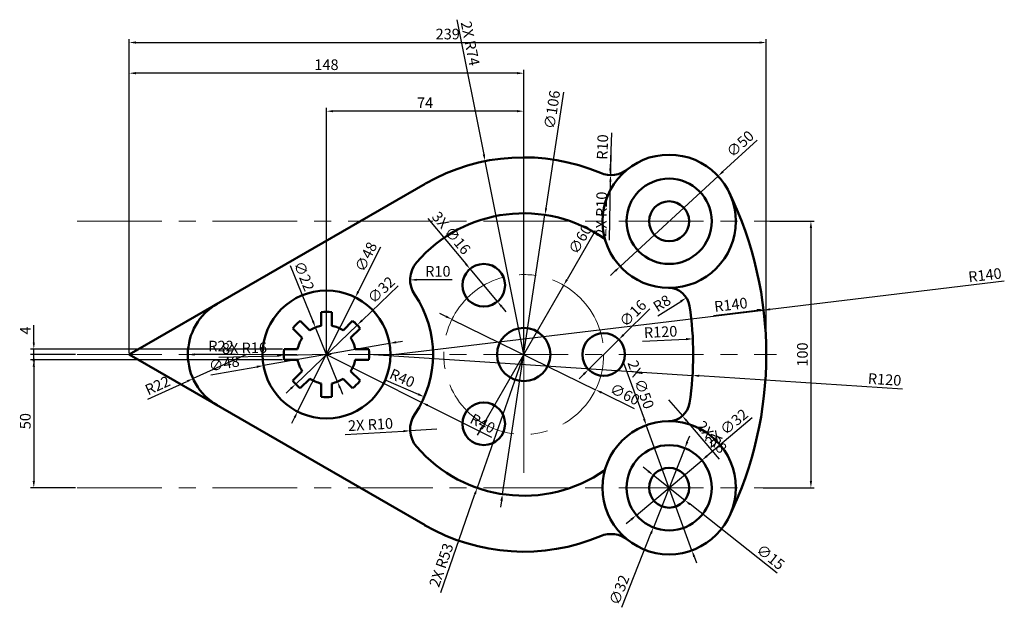
# Model space of a CAD drawing. Units: millimetres. Extents: x 2278 to 2648, y 1514 to 1735.
import ezdxf

# ---------------------------------------------------------------- set-up
doc = ezdxf.new("R2010")
doc.units = ezdxf.units.MM
doc.linetypes.add('CENTER', pattern=[50.8, 31.75, -6.35, 6.35, -6.35])
for name, color, linetype, lineweight in [('M-CNTR', 4, 'CENTER', 18), ('M-CONS', 8, 'Continuous', 13), ('M-DIMS', 2, 'Continuous', 25), ('M-OUTL', 7, 'Continuous', 50)]:
    doc.layers.add(name, color=color, linetype=linetype, lineweight=lineweight)
doc.styles.get("Standard").update_dxf_attribs({"font": 'arial.ttf'})
doc.dimstyles.new('ISO-25', dxfattribs={"dimtxt": 4, "dimasz": 2.5, "dimexe": 1.25, "dimexo": 0.625, "dimtad": 1, "dimtxsty": 'Standard', "dimcen": 2.5, "dimadec": 0, "dimazin": 0, "dimtfac": 1, "dimtmove": 0, "dimatfit": 3, "dimfxl": 1, "dimarcsym": 0})

# ---------------------------------------------------------------- blocks, each defined once
blk = doc.blocks.new('*D1')
at = {"layer": 'Defpoints', "color": 0, "transparency": 16777216}
for p in [(2393.46, 1700.37), (2393.46, 1609.04), (2467.46, 1609.04)]:
    blk.add_point(p, dxfattribs=at)
at = {"layer": 'M-DIMS', "color": 0, "lineweight": -2, "transparency": 16777216}
for p, q in [((2393.46, 1609.67), (2393.46, 1701.62)), ((2464.96, 1700.37), (2395.96, 1700.37)), ((2467.46, 1609.67), (2467.46, 1701.62))]:
    blk.add_line(p, q, dxfattribs=at)
at = {"layer": 'M-DIMS', "color": 0, "transparency": 16777216}
for points in [[(2395.96, 1700.78), (2395.96, 1699.95), (2393.46, 1700.37)], [(2464.96, 1700.78), (2464.96, 1699.95), (2467.46, 1700.37)]]:
    blk.add_solid(points, dxfattribs=at)
at = {"layer": 'M-DIMS', "color": 0, "transparency": 16777216, "insert": (2430.46, 1702.99), "char_height": 4, "attachment_point": 5}
blk.add_mtext('74', dxfattribs=at)
blk = doc.blocks.new('*D2')
at = {"layer": 'Defpoints', "color": 0, "transparency": 16777216}
for p in [(2319.46, 1714.62), (2319.46, 1669.34), (2467.46, 1609.04)]:
    blk.add_point(p, dxfattribs=at)
at = {"layer": 'M-DIMS', "color": 0, "lineweight": -2, "transparency": 16777216}
for p, q in [((2319.46, 1669.96), (2319.46, 1715.87)), ((2464.96, 1714.62), (2321.96, 1714.62)), ((2467.46, 1609.67), (2467.46, 1715.87))]:
    blk.add_line(p, q, dxfattribs=at)
at = {"layer": 'M-DIMS', "color": 0, "transparency": 16777216}
for points in [[(2321.96, 1715.04), (2321.96, 1714.21), (2319.46, 1714.62)], [(2464.96, 1715.04), (2464.96, 1714.21), (2467.46, 1714.62)]]:
    blk.add_solid(points, dxfattribs=at)
at = {"layer": 'M-DIMS', "color": 0, "transparency": 16777216, "insert": (2393.46, 1717.29), "char_height": 4, "attachment_point": 5}
blk.add_mtext('148', dxfattribs=at)
blk = doc.blocks.new('*D3')
at = {"layer": 'Defpoints', "color": 0, "transparency": 16777216}
for p in [(2404.27, 1630.47), (2382.64, 1587.62)]:
    blk.add_point(p, dxfattribs=at)
at = {"layer": 'M-DIMS', "color": 0, "lineweight": -2, "transparency": 16777216}
for p, q in [((2413.78, 1649.3), (2405.4, 1632.7)), ((2382.64, 1587.62), (2404.27, 1630.47)), ((2381.52, 1585.39), (2380.39, 1583.16))]:
    blk.add_line(p, q, dxfattribs=at)
at = {"layer": 'M-DIMS', "color": 0, "transparency": 16777216}
for points in [[(2405.03, 1632.89), (2405.77, 1632.51), (2404.27, 1630.47)], [(2381.14, 1585.58), (2381.89, 1585.2), (2382.64, 1587.62)]]:
    blk.add_solid(points, dxfattribs=at)
at = {"layer": 'M-DIMS', "color": 0, "transparency": 16777216, "insert": (2408.74, 1645.49), "char_height": 4, "attachment_point": 5, "rotation": 63.213}
blk.add_mtext('∅48', dxfattribs=at)
blk = doc.blocks.new('*D4')
at = {"layer": 'Defpoints', "color": 0, "transparency": 16777216}
for p in [(2405.01, 1620.12), (2381.91, 1597.97)]:
    blk.add_point(p, dxfattribs=at)
at = {"layer": 'M-DIMS', "color": 0, "lineweight": -2, "transparency": 16777216}
for p, q in [((2420.35, 1634.83), (2406.81, 1621.85)), ((2381.91, 1597.97), (2405.01, 1620.12)), ((2380.1, 1596.24), (2378.3, 1594.51))]:
    blk.add_line(p, q, dxfattribs=at)
at = {"layer": 'M-DIMS', "color": 0, "transparency": 16777216}
for points in [[(2406.52, 1622.15), (2407.1, 1621.55), (2405.01, 1620.12)], [(2379.82, 1596.54), (2380.39, 1595.94), (2381.91, 1597.97)]]:
    blk.add_solid(points, dxfattribs=at)
at = {"layer": 'M-DIMS', "color": 0, "transparency": 16777216, "insert": (2414.35, 1632.93), "char_height": 4, "attachment_point": 5, "rotation": 43.7976}
blk.add_mtext('∅32', dxfattribs=at)
blk = doc.blocks.new('*D5')
at = {"layer": 'Defpoints', "color": 0, "transparency": 16777216}
for p in [(2389.32, 1619.24), (2397.6, 1598.85)]:
    blk.add_point(p, dxfattribs=at)
at = {"layer": 'M-DIMS', "color": 0, "lineweight": -2, "transparency": 16777216}
for p, q in [((2379.87, 1642.49), (2388.38, 1621.55)), ((2397.6, 1598.85), (2389.32, 1619.24)), ((2398.54, 1596.54), (2399.48, 1594.22))]:
    blk.add_line(p, q, dxfattribs=at)
at = {"layer": 'M-DIMS', "color": 0, "transparency": 16777216}
for points in [[(2388.76, 1621.71), (2387.99, 1621.4), (2389.32, 1619.24)], [(2398.92, 1596.69), (2398.15, 1596.38), (2397.6, 1598.85)]]:
    blk.add_solid(points, dxfattribs=at)
at = {"layer": 'M-DIMS', "color": 0, "transparency": 16777216, "insert": (2384.57, 1638.3), "char_height": 4, "attachment_point": 5, "rotation": 292.1082}
blk.add_mtext('∅22', dxfattribs=at)
blk = doc.blocks.new('*D6')
at = {"layer": 'Defpoints', "color": 0, "transparency": 16777216}
for p in [(2440.52, 1622.24), (2494.4, 1595.85)]:
    blk.add_point(p, dxfattribs=at)
at = {"layer": 'M-DIMS', "color": 0, "lineweight": -2, "transparency": 16777216}
for p, q in [((2438.27, 1623.34), (2436.02, 1624.44)), ((2440.52, 1622.24), (2494.4, 1595.85)), ((2509.06, 1588.67), (2496.65, 1594.75))]:
    blk.add_line(p, q, dxfattribs=at)
at = {"layer": 'M-DIMS', "color": 0, "transparency": 16777216}
for points in [[(2438.45, 1623.71), (2438.09, 1622.96), (2440.52, 1622.24)], [(2496.83, 1595.13), (2496.46, 1594.38), (2494.4, 1595.85)]]:
    blk.add_solid(points, dxfattribs=at)
at = {"layer": 'M-DIMS', "color": 0, "transparency": 16777216, "insert": (2505.2, 1593.66), "char_height": 4, "attachment_point": 5, "rotation": 333.9087}
blk.add_mtext('∅60', dxfattribs=at)
blk = doc.blocks.new('*D7')
at = {"layer": 'Defpoints', "color": 0, "transparency": 16777216}
for p in [(2503.14, 1614.67), (2491.77, 1603.42)]:
    blk.add_point(p, dxfattribs=at)
at = {"layer": 'M-DIMS', "color": 0, "lineweight": -2, "transparency": 16777216}
for p, q in [((2514.75, 1626.16), (2504.92, 1616.43)), ((2491.77, 1603.42), (2503.14, 1614.67)), ((2490, 1601.66), (2488.22, 1599.9))]:
    blk.add_line(p, q, dxfattribs=at)
at = {"layer": 'M-DIMS', "color": 0, "transparency": 16777216}
for points in [[(2504.63, 1616.73), (2505.21, 1616.14), (2503.14, 1614.67)], [(2489.7, 1601.95), (2490.29, 1601.36), (2491.77, 1603.42)]]:
    blk.add_solid(points, dxfattribs=at)
at = {"layer": 'M-DIMS', "color": 0, "transparency": 16777216, "insert": (2508.77, 1624.15), "char_height": 4, "attachment_point": 5, "rotation": 44.7113}
blk.add_mtext('∅16', dxfattribs=at)
blk = doc.blocks.new('*D8')
at = {"layer": 'Defpoints', "color": 0, "transparency": 16777216}
for p in [(2540.39, 1676), (2503.64, 1642.09)]:
    blk.add_point(p, dxfattribs=at)
at = {"layer": 'M-DIMS', "color": 0, "lineweight": -2, "transparency": 16777216}
for p, q in [((2555.05, 1689.53), (2542.22, 1677.69)), ((2503.64, 1642.09), (2540.39, 1676)), ((2501.8, 1640.4), (2499.96, 1638.7))]:
    blk.add_line(p, q, dxfattribs=at)
at = {"layer": 'M-DIMS', "color": 0, "transparency": 16777216}
for points in [[(2541.94, 1678), (2542.51, 1677.39), (2540.39, 1676)], [(2501.52, 1640.7), (2502.08, 1640.09), (2503.64, 1642.09)]]:
    blk.add_solid(points, dxfattribs=at)
at = {"layer": 'M-DIMS', "color": 0, "transparency": 16777216, "insert": (2549.01, 1687.73), "char_height": 4, "attachment_point": 5, "rotation": 42.6936}
blk.add_mtext('∅50', dxfattribs=at)
blk = doc.blocks.new('*D9')
at = {"layer": 'Defpoints', "color": 0, "transparency": 16777216}
for p in [(2527.9, 1573.92), (2516.12, 1544.17)]:
    blk.add_point(p, dxfattribs=at)
at = {"layer": 'M-DIMS', "color": 0, "lineweight": -2, "transparency": 16777216}
for p, q in [((2528.82, 1576.25), (2529.74, 1578.57)), ((2527.9, 1573.92), (2516.12, 1544.17)), ((2504.27, 1514.22), (2515.2, 1541.84))]:
    blk.add_line(p, q, dxfattribs=at)
at = {"layer": 'M-DIMS', "color": 0, "transparency": 16777216}
for points in [[(2528.43, 1576.4), (2529.21, 1576.09), (2527.9, 1573.92)], [(2514.81, 1542), (2515.59, 1541.69), (2516.12, 1544.17)]]:
    blk.add_solid(points, dxfattribs=at)
at = {"layer": 'M-DIMS', "color": 0, "transparency": 16777216, "insert": (2503.76, 1520.49), "char_height": 4, "attachment_point": 5, "rotation": 68.4062}
blk.add_mtext('∅32', dxfattribs=at)
blk = doc.blocks.new('*D10')
at = {"layer": 'Defpoints', "color": 0, "transparency": 16777216}
for p in [(2516.13, 1563.71), (2527.89, 1554.38)]:
    blk.add_point(p, dxfattribs=at)
at = {"layer": 'M-DIMS', "color": 0, "lineweight": -2, "transparency": 16777216}
for p, q in [((2514.18, 1565.26), (2512.22, 1566.81)), ((2516.13, 1563.71), (2527.89, 1554.38)), ((2562.49, 1526.93), (2529.85, 1552.83))]:
    blk.add_line(p, q, dxfattribs=at)
at = {"layer": 'M-DIMS', "color": 0, "transparency": 16777216}
for points in [[(2514.44, 1565.59), (2513.92, 1564.93), (2516.13, 1563.71)], [(2530.1, 1553.16), (2529.59, 1552.5), (2527.89, 1554.38)]]:
    blk.add_solid(points, dxfattribs=at)
at = {"layer": 'M-DIMS', "color": 0, "transparency": 16777216, "insert": (2559.77, 1532.64), "char_height": 4, "attachment_point": 5, "rotation": 321.5765}
blk.add_mtext('∅15', dxfattribs=at)
blk = doc.blocks.new('*D11')
at = {"layer": 'Defpoints', "color": 0, "transparency": 16777216}
for p in [(2393.46, 1609.04), (2430.16, 1593.14)]:
    blk.add_point(p, dxfattribs=at)
at = {"layer": 'M-DIMS', "color": 0, "lineweight": -2, "transparency": 16777216}
blk.add_line((2415.67, 1599.42), (2427.87, 1594.14), dxfattribs=at)
at = {"layer": 'M-DIMS', "color": 0, "transparency": 16777216}
blk.add_solid([(2428.03, 1594.52), (2427.7, 1593.76), (2430.16, 1593.14)], dxfattribs=at)
at = {"layer": 'M-DIMS', "color": 0, "transparency": 16777216, "insert": (2421.68, 1599.72), "char_height": 4, "attachment_point": 5, "rotation": 336.5775}
blk.add_mtext('R40', dxfattribs=at)
blk = doc.blocks.new('*D12')
at = {"layer": 'Defpoints', "color": 0, "transparency": 16777216}
for p in [(2557.42, 1626.02), (2418.45, 1609.04)]:
    blk.add_point(p, dxfattribs=at)
at = {"layer": 'M-DIMS', "color": 0, "lineweight": -2, "transparency": 16777216}
blk.add_line((2538.65, 1623.73), (2554.93, 1625.72), dxfattribs=at)
at = {"layer": 'M-DIMS', "color": 0, "transparency": 16777216}
blk.add_solid([(2554.88, 1626.13), (2554.99, 1625.3), (2557.42, 1626.02)], dxfattribs=at)
at = {"layer": 'M-DIMS', "color": 0, "transparency": 16777216, "insert": (2545.23, 1627.22), "char_height": 4, "attachment_point": 5, "rotation": 6.9648}
blk.add_mtext('R140', dxfattribs=at)
blk = doc.blocks.new('*D13')
at = {"layer": 'Defpoints', "color": 0, "transparency": 16777216}
for p in [(2530.91, 1614.93), (2411.05, 1609.04)]:
    blk.add_point(p, dxfattribs=at)
at = {"layer": 'M-DIMS', "color": 0, "lineweight": -2, "transparency": 16777216}
blk.add_line((2512.03, 1614.01), (2528.41, 1614.81), dxfattribs=at)
at = {"layer": 'M-DIMS', "color": 0, "transparency": 16777216}
blk.add_solid([(2528.39, 1615.23), (2528.43, 1614.4), (2530.91, 1614.93)], dxfattribs=at)
at = {"layer": 'M-DIMS', "color": 0, "transparency": 16777216, "insert": (2518.84, 1617.01), "char_height": 4, "attachment_point": 5, "rotation": 2.8132}
blk.add_mtext('R120', dxfattribs=at)
blk = doc.blocks.new('*D14')
at = {"layer": 'Defpoints', "color": 0, "transparency": 16777216}
for p in [(2528.5, 1630.34), (2521.76, 1626.05)]:
    blk.add_point(p, dxfattribs=at)
at = {"layer": 'M-DIMS', "color": 0, "lineweight": -2, "transparency": 16777216}
blk.add_line((2517.78, 1623.52), (2526.4, 1629), dxfattribs=at)
at = {"layer": 'M-DIMS', "color": 0, "transparency": 16777216}
blk.add_solid([(2526.17, 1629.35), (2526.62, 1628.65), (2528.5, 1630.34)], dxfattribs=at)
at = {"layer": 'M-DIMS', "color": 0, "transparency": 16777216, "insert": (2519.6, 1627.84), "char_height": 4, "attachment_point": 5, "rotation": 32.4759}
blk.add_mtext('R8', dxfattribs=at)
blk = doc.blocks.new('*D15')
at = {"layer": 'Defpoints', "color": 0, "transparency": 16777216}
for p in [(2475.43, 1661.44), (2459.49, 1556.65)]:
    blk.add_point(p, dxfattribs=at)
at = {"layer": 'M-DIMS', "color": 0, "lineweight": -2, "transparency": 16777216}
for p, q in [((2482.44, 1707.55), (2475.8, 1663.91)), ((2459.49, 1556.65), (2475.43, 1661.44)), ((2459.11, 1554.18), (2458.74, 1551.7))]:
    blk.add_line(p, q, dxfattribs=at)
at = {"layer": 'M-DIMS', "color": 0, "transparency": 16777216}
for points in [[(2475.39, 1663.98), (2476.22, 1663.85), (2475.43, 1661.44)], [(2458.7, 1554.24), (2459.52, 1554.11), (2459.49, 1556.65)]]:
    blk.add_solid(points, dxfattribs=at)
at = {"layer": 'M-DIMS', "color": 0, "transparency": 16777216, "insert": (2478.61, 1700.84), "char_height": 4, "attachment_point": 5, "rotation": 81.3508}
blk.add_mtext('∅106', dxfattribs=at)
blk = doc.blocks.new('*D16')
at = {"layer": 'Defpoints', "color": 0, "transparency": 16777216}
for p in [(2500.19, 1686.41), (2499.86, 1676.41)]:
    blk.add_point(p, dxfattribs=at)
at = {"layer": 'M-DIMS', "color": 0, "lineweight": -2, "transparency": 16777216}
blk.add_line((2500.38, 1692.2), (2499.94, 1678.91), dxfattribs=at)
at = {"layer": 'M-DIMS', "color": 0, "transparency": 16777216}
blk.add_solid([(2499.52, 1678.92), (2500.35, 1678.9), (2499.86, 1676.41)], dxfattribs=at)
at = {"layer": 'M-DIMS', "color": 0, "transparency": 16777216, "insert": (2497.53, 1686.89), "char_height": 4, "attachment_point": 5, "rotation": 88.1053}
blk.add_mtext('R10', dxfattribs=at)
blk = doc.blocks.new('*D17')
at = {"layer": 'Defpoints', "color": 0, "transparency": 16777216}
for p in [(2424.86, 1637.07), (2434.86, 1637.08)]:
    blk.add_point(p, dxfattribs=at)
at = {"layer": 'M-DIMS', "color": 0, "lineweight": -2, "transparency": 16777216}
blk.add_line((2440.65, 1637.09), (2427.36, 1637.07), dxfattribs=at)
at = {"layer": 'M-DIMS', "color": 0, "transparency": 16777216}
blk.add_solid([(2427.36, 1637.49), (2427.36, 1636.66), (2424.86, 1637.07)], dxfattribs=at)
at = {"layer": 'M-DIMS', "color": 0, "transparency": 16777216, "insert": (2435.25, 1639.75), "char_height": 4, "attachment_point": 5, "rotation": 0.0789}
blk.add_mtext('R10', dxfattribs=at)
blk = doc.blocks.new('*D18')
at = {"layer": 'Defpoints', "color": 0, "transparency": 16777216}
for p in [(2559.19, 1659.04), (2556.66, 1559.04), (2575.21, 1559.04)]:
    blk.add_point(p, dxfattribs=at)
at = {"layer": 'M-DIMS', "color": 0, "lineweight": -2, "transparency": 16777216}
for p, q in [((2559.82, 1659.04), (2576.46, 1659.04)), ((2575.21, 1656.54), (2575.21, 1561.54)), ((2557.29, 1559.04), (2576.46, 1559.04))]:
    blk.add_line(p, q, dxfattribs=at)
at = {"layer": 'M-DIMS', "color": 0, "transparency": 16777216}
for points in [[(2574.79, 1656.54), (2575.63, 1656.54), (2575.21, 1659.04)], [(2574.79, 1561.54), (2575.63, 1561.54), (2575.21, 1559.04)]]:
    blk.add_solid(points, dxfattribs=at)
at = {"layer": 'M-DIMS', "color": 0, "transparency": 16777216, "insert": (2572.54, 1609.04), "char_height": 4, "attachment_point": 5, "rotation": 90}
blk.add_mtext('100', dxfattribs=at)
blk = doc.blocks.new('*D19')
at = {"layer": 'Defpoints', "color": 0, "transparency": 16777216}
for p in [(2341.46, 1609.04), (2363.46, 1609.04)]:
    blk.add_point(p, dxfattribs=at)
at = {"layer": 'M-DIMS', "color": 0, "lineweight": -2, "transparency": 16777216}
blk.add_line((2359.28, 1609.04), (2343.96, 1609.04), dxfattribs=at)
at = {"layer": 'M-DIMS', "color": 0, "transparency": 16777216}
blk.add_solid([(2343.96, 1609.46), (2343.96, 1608.63), (2341.46, 1609.04)], dxfattribs=at)
at = {"layer": 'M-DIMS', "color": 0, "transparency": 16777216, "insert": (2353.89, 1611.68), "char_height": 4, "attachment_point": 5}
blk.add_mtext('R22', dxfattribs=at)
blk = doc.blocks.new('BOSS-D50-D32-BORE15')
for radius in [25, 16, 7.5]:
    blk.add_circle((0, 0), radius)
blk = doc.blocks.new('HOLE-D16')
blk.add_circle((0, 0), 8)
blk = doc.blocks.new('*D22')
at = {"layer": 'Defpoints', "color": 0, "transparency": 16777216}
for p in [(2558.45, 1726.13), (2319.46, 1609.04), (2558.45, 1609.04)]:
    blk.add_point(p, dxfattribs=at)
at = {"layer": 'M-DIMS', "color": 0, "lineweight": -2, "transparency": 16777216}
for p, q in [((2319.46, 1609.67), (2319.46, 1727.38)), ((2321.96, 1726.13), (2555.95, 1726.13)), ((2558.45, 1609.67), (2558.45, 1727.38))]:
    blk.add_line(p, q, dxfattribs=at)
at = {"layer": 'M-DIMS', "color": 0, "transparency": 16777216}
for points in [[(2321.96, 1726.55), (2321.96, 1725.72), (2319.46, 1726.13)], [(2555.95, 1726.55), (2555.95, 1725.72), (2558.45, 1726.13)]]:
    blk.add_solid(points, dxfattribs=at)
at = {"layer": 'M-DIMS', "color": 0, "transparency": 16777216, "insert": (2438.95, 1728.8), "char_height": 4, "attachment_point": 5}
blk.add_mtext('239', dxfattribs=at)
blk = doc.blocks.new('*D23')
at = {"layer": 'Defpoints', "color": 0, "transparency": 16777216}
for p in [(2283.66, 1611.04), (2377.58, 1611.04), (2377.58, 1607.04)]:
    blk.add_point(p, dxfattribs=at)
at = {"layer": 'M-DIMS', "color": 0, "lineweight": -2, "transparency": 16777216}
for p, q in [((2283.66, 1613.54), (2283.66, 1620.06)), ((2376.96, 1611.04), (2282.41, 1611.04)), ((2283.66, 1607.04), (2283.66, 1611.04)), ((2376.96, 1607.04), (2282.41, 1607.04)), ((2283.66, 1604.54), (2283.66, 1602.04))]:
    blk.add_line(p, q, dxfattribs=at)
at = {"layer": 'M-DIMS', "color": 0, "transparency": 16777216}
for points in [[(2283.25, 1613.54), (2284.08, 1613.54), (2283.66, 1611.04)], [(2283.25, 1604.54), (2284.08, 1604.54), (2283.66, 1607.04)]]:
    blk.add_solid(points, dxfattribs=at)
at = {"layer": 'M-DIMS', "color": 0, "transparency": 16777216, "insert": (2281.04, 1618.05), "char_height": 4, "attachment_point": 5, "rotation": 90}
blk.add_mtext('4', dxfattribs=at)
blk = doc.blocks.new('*D24')
at = {"layer": 'Defpoints', "color": 0, "transparency": 16777216}
for p in [(2299.96, 1609.04), (2283.66, 1559.04), (2299.96, 1559.04)]:
    blk.add_point(p, dxfattribs=at)
at = {"layer": 'M-DIMS', "color": 0, "lineweight": -2, "transparency": 16777216}
for p, q in [((2299.34, 1609.04), (2282.41, 1609.04)), ((2283.66, 1606.54), (2283.66, 1561.54)), ((2299.34, 1559.04), (2282.41, 1559.04))]:
    blk.add_line(p, q, dxfattribs=at)
at = {"layer": 'M-DIMS', "color": 0, "transparency": 16777216}
for points in [[(2283.25, 1606.54), (2284.08, 1606.54), (2283.66, 1609.04)], [(2283.25, 1561.54), (2284.08, 1561.54), (2283.66, 1559.04)]]:
    blk.add_solid(points, dxfattribs=at)
at = {"layer": 'M-DIMS', "color": 0, "transparency": 16777216, "insert": (2281, 1584.04), "char_height": 4, "attachment_point": 5, "rotation": 90}
blk.add_mtext('50', dxfattribs=at)
blk = doc.blocks.new('*D25')
at = {"layer": 'Defpoints', "color": 0, "transparency": 16777216}
for p in [(2453, 1681.62), (2467.46, 1609.04)]:
    blk.add_point(p, dxfattribs=at)
at = {"layer": 'M-DIMS', "color": 0, "lineweight": -2, "transparency": 16777216}
for p, q in [((2442.43, 1734.7), (2452.51, 1684.07)), ((2467.46, 1609.04), (2453, 1681.62))]:
    blk.add_line(p, q, dxfattribs=at)
at = {"layer": 'M-DIMS', "color": 0, "transparency": 16777216}
blk.add_solid([(2452.92, 1684.15), (2452.1, 1683.99), (2453, 1681.62)], dxfattribs=at)
at = {"layer": 'M-DIMS', "color": 0, "transparency": 16777216, "insert": (2446.91, 1725.68), "char_height": 4, "attachment_point": 5, "rotation": 281.2666}
blk.add_mtext('2X R74', dxfattribs=at)
blk = doc.blocks.new('*D26')
at = {"layer": 'Defpoints', "color": 0, "transparency": 16777216}
for p in [(2557.45, 1625.7), (2418.45, 1609.04)]:
    blk.add_point(p, dxfattribs=at)
at = {"layer": 'M-DIMS', "color": 0, "lineweight": -2, "transparency": 16777216}
for p, q in [((2647.76, 1636.52), (2559.94, 1626)), ((2418.45, 1609.04), (2557.45, 1625.7))]:
    blk.add_line(p, q, dxfattribs=at)
at = {"layer": 'M-DIMS', "color": 0, "transparency": 16777216}
blk.add_solid([(2559.89, 1626.41), (2559.99, 1625.58), (2557.45, 1625.7)], dxfattribs=at)
at = {"layer": 'M-DIMS', "color": 0, "transparency": 16777216, "insert": (2640.54, 1638.34), "char_height": 4, "attachment_point": 5, "rotation": 6.8327}
blk.add_mtext('R140', dxfattribs=at)
blk = doc.blocks.new('*D27')
at = {"layer": 'Defpoints', "color": 0, "transparency": 16777216}
for p in [(2411.05, 1609.04), (2530.8, 1601.2)]:
    blk.add_point(p, dxfattribs=at)
at = {"layer": 'M-DIMS', "color": 0, "lineweight": -2, "transparency": 16777216}
for p, q in [((2411.05, 1609.04), (2530.8, 1601.2)), ((2609.58, 1596.04), (2533.29, 1601.04))]:
    blk.add_line(p, q, dxfattribs=at)
at = {"layer": 'M-DIMS', "color": 0, "transparency": 16777216}
blk.add_solid([(2533.32, 1601.45), (2533.26, 1600.62), (2530.8, 1601.2)], dxfattribs=at)
at = {"layer": 'M-DIMS', "color": 0, "transparency": 16777216, "insert": (2602.82, 1599.16), "char_height": 4, "attachment_point": 5, "rotation": 356.2519}
blk.add_mtext('R120', dxfattribs=at)
blk = doc.blocks.new('*D28')
at = {"layer": 'Defpoints', "color": 0, "transparency": 16777216}
for p in [(2467.46, 1609.04), (2450, 1559)]:
    blk.add_point(p, dxfattribs=at)
at = {"layer": 'M-DIMS', "color": 0, "lineweight": -2, "transparency": 16777216}
for p, q in [((2467.46, 1609.04), (2450, 1559)), ((2436.33, 1519.78), (2449.18, 1556.64))]:
    blk.add_line(p, q, dxfattribs=at)
at = {"layer": 'M-DIMS', "color": 0, "transparency": 16777216}
blk.add_solid([(2448.79, 1556.78), (2449.57, 1556.5), (2450, 1559)], dxfattribs=at)
at = {"layer": 'M-DIMS', "color": 0, "transparency": 16777216, "insert": (2437.01, 1529.85), "char_height": 4, "attachment_point": 5, "rotation": 70.7723}
blk.add_mtext('2X R53', dxfattribs=at)
blk = doc.blocks.new('*D29')
at = {"layer": 'Defpoints', "color": 0, "transparency": 16777216}
for p in [(2393.46, 1609.04), (2429.2, 1591.09)]:
    blk.add_point(p, dxfattribs=at)
at = {"layer": 'M-DIMS', "color": 0, "lineweight": -2, "transparency": 16777216}
for p, q in [((2393.46, 1609.04), (2429.2, 1591.09)), ((2455.47, 1577.9), (2431.44, 1589.97))]:
    blk.add_line(p, q, dxfattribs=at)
at = {"layer": 'M-DIMS', "color": 0, "transparency": 16777216}
blk.add_solid([(2431.62, 1590.34), (2431.25, 1589.6), (2429.2, 1591.09)], dxfattribs=at)
at = {"layer": 'M-DIMS', "color": 0, "transparency": 16777216, "insert": (2451.85, 1582.71), "char_height": 4, "attachment_point": 5, "rotation": 333.3343}
blk.add_mtext('R40', dxfattribs=at)
blk = doc.blocks.new('*D30')
at = {"layer": 'Defpoints', "color": 0, "transparency": 16777216}
for p in [(2363.46, 1609.04), (2343.41, 1600)]:
    blk.add_point(p, dxfattribs=at)
at = {"layer": 'M-DIMS', "color": 0, "lineweight": -2, "transparency": 16777216}
for p, q in [((2363.46, 1609.04), (2343.41, 1600)), ((2326.47, 1592.35), (2341.13, 1598.97))]:
    blk.add_line(p, q, dxfattribs=at)
at = {"layer": 'M-DIMS', "color": 0, "transparency": 16777216}
blk.add_solid([(2340.95, 1599.35), (2341.3, 1598.59), (2343.41, 1600)], dxfattribs=at)
at = {"layer": 'M-DIMS', "color": 0, "transparency": 16777216, "insert": (2330.29, 1596.97), "char_height": 4, "attachment_point": 5, "rotation": 24.287}
blk.add_mtext('R22', dxfattribs=at)
blk = doc.blocks.new('*D31')
at = {"layer": 'Defpoints', "color": 0, "transparency": 16777216}
for p in [(2434.86, 1581.01), (2424.87, 1580.43)]:
    blk.add_point(p, dxfattribs=at)
at = {"layer": 'M-DIMS', "color": 0, "lineweight": -2, "transparency": 16777216}
for p, q in [((2434.86, 1581.01), (2424.87, 1580.43)), ((2400.46, 1579.03), (2422.38, 1580.29))]:
    blk.add_line(p, q, dxfattribs=at)
at = {"layer": 'M-DIMS', "color": 0, "transparency": 16777216}
blk.add_solid([(2422.35, 1580.7), (2422.4, 1579.87), (2424.87, 1580.43)], dxfattribs=at)
at = {"layer": 'M-DIMS', "color": 0, "transparency": 16777216, "insert": (2410.02, 1582.25), "char_height": 4, "attachment_point": 5, "rotation": 3.2917}
blk.add_mtext('2X R10', dxfattribs=at)
blk = doc.blocks.new('*D32')
at = {"layer": 'Defpoints', "color": 0, "transparency": 16777216}
for p in [(2521.76, 1592.04), (2526.99, 1585.99)]:
    blk.add_point(p, dxfattribs=at)
at = {"layer": 'M-DIMS', "color": 0, "lineweight": -2, "transparency": 16777216}
for p, q in [((2521.76, 1592.04), (2526.99, 1585.99)), ((2540.97, 1569.83), (2528.62, 1584.1))]:
    blk.add_line(p, q, dxfattribs=at)
at = {"layer": 'M-DIMS', "color": 0, "transparency": 16777216}
blk.add_solid([(2528.94, 1584.37), (2528.31, 1583.83), (2526.99, 1585.99)], dxfattribs=at)
at = {"layer": 'M-DIMS', "color": 0, "transparency": 16777216, "insert": (2537.63, 1577.76), "char_height": 4, "attachment_point": 5, "rotation": 310.8555}
blk.add_mtext('2X R8', dxfattribs=at)
blk = doc.blocks.new('*D33')
at = {"layer": 'Defpoints', "color": 0, "transparency": 16777216}
for p in [(2500.19, 1686.41), (2500.03, 1676.41)]:
    blk.add_point(p, dxfattribs=at)
at = {"layer": 'M-DIMS', "color": 0, "lineweight": -2, "transparency": 16777216}
for p, q in [((2500.19, 1686.41), (2500.03, 1676.41)), ((2499.64, 1651.95), (2499.99, 1673.91))]:
    blk.add_line(p, q, dxfattribs=at)
at = {"layer": 'M-DIMS', "color": 0, "transparency": 16777216}
blk.add_solid([(2499.57, 1673.91), (2500.41, 1673.9), (2500.03, 1676.41)], dxfattribs=at)
at = {"layer": 'M-DIMS', "color": 0, "transparency": 16777216, "insert": (2497.13, 1661.72), "char_height": 4, "attachment_point": 5, "rotation": 89.099}
blk.add_mtext('2X R10', dxfattribs=at)
blk = doc.blocks.new('*D34')
at = {"layer": 'Defpoints', "color": 0, "transparency": 16777216}
for p in [(2482.46, 1635.03), (2452.46, 1583.06)]:
    blk.add_point(p, dxfattribs=at)
at = {"layer": 'M-DIMS', "color": 0, "lineweight": -2, "transparency": 16777216}
for p, q in [((2494.29, 1655.52), (2483.71, 1637.19)), ((2452.46, 1583.06), (2482.46, 1635.03)), ((2451.21, 1580.9), (2449.96, 1578.73))]:
    blk.add_line(p, q, dxfattribs=at)
at = {"layer": 'M-DIMS', "color": 0, "transparency": 16777216}
for points in [[(2483.35, 1637.4), (2484.07, 1636.98), (2482.46, 1635.03)], [(2450.85, 1581.11), (2451.57, 1580.69), (2452.46, 1583.06)]]:
    blk.add_solid(points, dxfattribs=at)
at = {"layer": 'M-DIMS', "color": 0, "transparency": 16777216, "insert": (2489.05, 1652), "char_height": 4, "attachment_point": 5, "rotation": 60.0006}
blk.add_mtext('∅60', dxfattribs=at)
blk = doc.blocks.new('*D35')
at = {"layer": 'Defpoints', "color": 0, "transparency": 16777216}
for p in [(2447.32, 1641.15), (2457.6, 1628.9)]:
    blk.add_point(p, dxfattribs=at)
at = {"layer": 'M-DIMS', "color": 0, "lineweight": -2, "transparency": 16777216}
for p, q in [((2431.43, 1660.08), (2445.71, 1643.07)), ((2457.6, 1628.9), (2447.32, 1641.15)), ((2459.21, 1626.98), (2460.81, 1625.07))]:
    blk.add_line(p, q, dxfattribs=at)
at = {"layer": 'M-DIMS', "color": 0, "transparency": 16777216}
for points in [[(2446.03, 1643.34), (2445.39, 1642.8), (2447.32, 1641.15)], [(2459.53, 1627.25), (2458.89, 1626.71), (2457.6, 1628.9)]]:
    blk.add_solid(points, dxfattribs=at)
at = {"layer": 'M-DIMS', "color": 0, "transparency": 16777216, "insert": (2439.9, 1654.32), "char_height": 4, "attachment_point": 5, "rotation": 309.997}
blk.add_mtext('3X ∅16', dxfattribs=at)
blk = doc.blocks.new('*D36')
at = {"layer": 'Defpoints', "color": 0, "transparency": 16777216}
for p in [(2513.46, 1582.54), (2530.56, 1535.55)]:
    blk.add_point(p, dxfattribs=at)
at = {"layer": 'M-DIMS', "color": 0, "lineweight": -2, "transparency": 16777216}
for p, q in [((2504.95, 1605.92), (2512.6, 1584.89)), ((2530.56, 1535.55), (2513.46, 1582.54)), ((2531.42, 1533.2), (2532.27, 1530.85))]:
    blk.add_line(p, q, dxfattribs=at)
at = {"layer": 'M-DIMS', "color": 0, "transparency": 16777216}
for points in [[(2513, 1585.03), (2512.21, 1584.74), (2513.46, 1582.54)], [(2531.81, 1533.35), (2531.02, 1533.06), (2530.56, 1535.55)]]:
    blk.add_solid(points, dxfattribs=at)
at = {"layer": 'M-DIMS', "color": 0, "transparency": 16777216, "insert": (2510.94, 1597.58), "char_height": 4, "attachment_point": 5, "rotation": 290.0004}
blk.add_mtext('2X ∅50', dxfattribs=at)
blk = doc.blocks.new('*D37')
at = {"layer": 'Defpoints', "color": 0, "transparency": 16777216}
for p in [(2534.27, 1569.33), (2509.75, 1548.76)]:
    blk.add_point(p, dxfattribs=at)
at = {"layer": 'M-DIMS', "color": 0, "lineweight": -2, "transparency": 16777216}
for p, q in [((2553.22, 1585.23), (2536.18, 1570.94)), ((2509.75, 1548.76), (2534.27, 1569.33)), ((2507.84, 1547.15), (2505.92, 1545.55))]:
    blk.add_line(p, q, dxfattribs=at)
at = {"layer": 'M-DIMS', "color": 0, "transparency": 16777216}
for points in [[(2535.91, 1571.26), (2536.45, 1570.62), (2534.27, 1569.33)], [(2507.57, 1547.47), (2508.11, 1546.83), (2509.75, 1548.76)]]:
    blk.add_solid(points, dxfattribs=at)
at = {"layer": 'M-DIMS', "color": 0, "transparency": 16777216, "insert": (2543.87, 1581.02), "char_height": 4, "attachment_point": 5, "rotation": 40.0008}
blk.add_mtext('2X ∅32', dxfattribs=at)
blk = doc.blocks.new('*D38')
at = {"layer": 'Defpoints', "color": 0, "transparency": 16777216}
for p in [(2417.09, 1613.21), (2369.82, 1604.88)]:
    blk.add_point(p, dxfattribs=at)
at = {"layer": 'M-DIMS', "color": 0, "lineweight": -2, "transparency": 16777216}
for p, q in [((2417.09, 1613.21), (2369.82, 1604.88)), ((2419.56, 1613.65), (2422.02, 1614.08)), ((2350.06, 1601.39), (2367.36, 1604.44))]:
    blk.add_line(p, q, dxfattribs=at)
at = {"layer": 'M-DIMS', "color": 0, "transparency": 16777216}
for points in [[(2419.48, 1614.06), (2419.63, 1613.24), (2417.09, 1613.21)], [(2367.29, 1604.85), (2367.43, 1604.03), (2369.82, 1604.88)]]:
    blk.add_solid(points, dxfattribs=at)
at = {"layer": 'M-DIMS', "color": 0, "transparency": 16777216, "insert": (2355.16, 1605.11), "char_height": 4, "attachment_point": 5, "rotation": 9.999}
blk.add_mtext('∅48', dxfattribs=at)
blk = doc.blocks.new('*D39')
at = {"layer": 'Defpoints', "color": 0, "transparency": 16777216}
for p in [(2377.46, 1608.65), (2393.46, 1609.04)]:
    blk.add_point(p, dxfattribs=at)
at = {"layer": 'M-DIMS', "color": 0, "lineweight": -2, "transparency": 16777216}
for p, q in [((2353.06, 1608.05), (2374.96, 1608.59)), ((2393.46, 1609.04), (2377.46, 1608.65))]:
    blk.add_line(p, q, dxfattribs=at)
at = {"layer": 'M-DIMS', "color": 0, "transparency": 16777216}
blk.add_solid([(2374.95, 1609.01), (2374.97, 1608.17), (2377.46, 1608.65)], dxfattribs=at)
at = {"layer": 'M-DIMS', "color": 0, "transparency": 16777216, "insert": (2362.7, 1610.96), "char_height": 4, "attachment_point": 5, "rotation": 1.4077}
blk.add_mtext('8X R16', dxfattribs=at)

msp = doc.modelspace()

# ---------------------------------------------------------------- linework, layer by layer
at = {"layer": 'M-CNTR'}
for p, q in [((2299.963, 1659.045), (2562.293, 1659.045)), ((2299.963, 1609.045), (2562.293, 1609.045)), ((2299.963, 1559.045), (2562.293, 1559.045))]:
    msp.add_line(p, q, dxfattribs=at)
msp.add_circle((2467.458, 1609.045), 30, dxfattribs=at)
at = {"layer": 'M-CONS'}
for p, q in [((2319.458, 1709.833), (2319.458, 1609.045)), ((2467.458, 1609.045), (2467.458, 1564.616))]:
    msp.add_line(p, q, dxfattribs=at)
at = {"layer": 'M-OUTL'}
for p, q in [((2319.458, 1609.045), (2430.458, 1673.13)), ((2383.647, 1621.684), (2387.224, 1618.107)), ((2391.458, 1624.919), (2391.458, 1619.861)), ((2395.458, 1624.919), (2395.458, 1619.861)), ((2403.269, 1621.684), (2399.692, 1618.107)), ((2380.819, 1618.855), (2384.395, 1615.279)), ((2406.097, 1618.855), (2402.521, 1615.279)), ((2377.583, 1611.045), (2382.641, 1611.045)), ((2409.332, 1611.045), (2404.275, 1611.045)), ((2319.458, 1609.045), (2430.458, 1544.959)), ((2377.583, 1607.045), (2382.641, 1607.045)), ((2409.332, 1607.045), (2404.275, 1607.045)), ((2380.819, 1599.234), (2384.395, 1602.81)), ((2383.647, 1596.405), (2387.224, 1599.982)), ((2403.269, 1596.405), (2399.692, 1599.982)), ((2406.097, 1599.234), (2402.521, 1602.81)), ((2391.458, 1593.17), (2391.458, 1598.228)), ((2395.458, 1593.17), (2395.458, 1598.228))]:
    msp.add_line(p, q, dxfattribs=at)
for centre, radius in [((2393.458, 1609.045), 24), ((2467.458, 1609.045), 10)]:
    msp.add_circle(centre, radius, dxfattribs=at)
for centre, radius, start, end in [((2467.458, 1609.045), 74, 67.06923, 119.84066), ((2500.186, 1686.407), 10, 247.06923, 308.57692), ((2418.449, 1609.045), 140, 334.22854, 25.77146), ((2467.458, 1609.045), 53, 54.9412, 139.30322), ((2434.857, 1637.083), 10, 139.30322, 214.10893), ((2521.756, 1626.046), 8, 8.73093, 89.55775), ((2393.458, 1609.045), 40, 325.89107, 34.10893), ((2363.458, 1609.045), 22, 120, 240), ((2411.054, 1609.045), 120, 351.26907, 8.73093), ((2393.458, 1609.045), 16, 127.81924, 142.18076), ((2393.458, 1609.045), 16, 82.81924, 97.18076), ((2393.458, 1609.045), 16, 37.81924, 52.18076), ((2393.458, 1609.045), 11, 100.47568, 124.52432), ((2393.458, 1609.045), 11, 55.47568, 79.52432), ((2393.458, 1609.045), 11, 145.47568, 169.52432), ((2393.458, 1609.045), 11, 10.47568, 34.52432), ((2393.458, 1609.045), 16, 172.81924, 187.18076), ((2393.458, 1609.045), 16, 352.81924, 7.18076), ((2393.458, 1609.045), 11, 190.47568, 214.52432), ((2393.458, 1609.045), 11, 325.47568, 349.52432), ((2393.458, 1609.045), 11, 235.47568, 259.52432), ((2393.458, 1609.045), 11, 280.47568, 304.52432), ((2393.458, 1609.045), 16, 217.81924, 232.18076), ((2393.458, 1609.045), 16, 307.81924, 322.18076), ((2393.458, 1609.045), 16, 262.81924, 277.18076), ((2521.756, 1592.044), 8, 270.44225, 351.26907), ((2434.857, 1581.006), 10, 145.89107, 220.69678), ((2467.458, 1609.045), 53, 220.69678, 305.0588), ((2467.458, 1609.045), 74, 239.84091, 292.93077), ((2500.186, 1531.683), 10, 51.42308, 112.93077)]:
    msp.add_arc(centre, radius, start, end, dxfattribs=at)

# ---------------------------------------------------------------- block references
for name, p in [('BOSS-D50-D32-BORE15', (2522.011, 1659.045)), ('HOLE-D16', (2452.458, 1635.025)), ('HOLE-D16', (2497.458, 1609.045)), ('HOLE-D16', (2452.458, 1583.064))]:
    msp.add_blockref(name, p, dxfattribs=at)
at = {"layer": 'M-OUTL', "rotation": 90}
msp.add_blockref('BOSS-D50-D32-BORE15', (2522.011, 1559.045), dxfattribs=at)

# ---------------------------------------------------------------- dimensions: what is measured, and where the dimension line sits
at = {"layer": 'M-DIMS'}
for mpoint, picture, middle in [((2453, 1681.619), '*D25', (2444.326, 1725.163)), ((2450.004, 1559.001), '*D28', (2439.531, 1528.975))]:
    dim = msp.add_radius_dim(center=(2467.458, 1609.045), mpoint=mpoint, text='2X <>', dimstyle='ISO-25', override={"dimdec": 0, "dimlfac": 1, "dimrnd": 0, "dimzin": 0, "dimdsep": 46, "dimlunit": 2}, dxfattribs=at)
    dim.commit()
    dim.dimension.update_dxf_attribs({"geometry": picture, "text_midpoint": middle, "dimtype": 164})
for base, p1, p2, override, picture, middle in [((2558.449, 1726.133), (2319.458, 1609.045), (2558.449, 1609.045), {"dimdec": 0, "dimlfac": 1, "dimrnd": 0, "dimzin": 0, "dimdsep": 46, "dimlunit": 2}, '*D22', (2438.954, 1728.802)), ((2319.458, 1714.623), (2467.458, 1609.045), (2319.458, 1669.339), {"dimclrd": 0, "dimclre": 0, "dimclrt": 0}, '*D2', (2393.458, 1717.29)), ((2393.458, 1700.365), (2467.458, 1609.045), (2393.458, 1609.045), {"dimclrd": 0, "dimclre": 0, "dimclrt": 0}, '*D1', (2430.458, 1702.99))]:
    dim = msp.add_linear_dim(base=base, p1=p1, p2=p2, dimstyle='ISO-25', override=override, dxfattribs=at)
    dim.commit()
    dim.dimension.update_dxf_attribs({"geometry": picture, "text_midpoint": middle})
for p1, p2, override, picture, middle in [((2459.488, 1556.647), (2475.428, 1661.442), {"dimclrd": 0, "dimclre": 0, "dimclrt": 0}, '*D15', (2481.357, 1700.418)), ((2503.636, 1642.093), (2540.385, 1675.997), {"dimclrd": 0, "dimclre": 0, "dimclrt": 0}, '*D8', (2550.894, 1685.692)), ((2452.458, 1583.064), (2482.458, 1635.026), {"dimdec": 0, "dimlfac": 1, "dimrnd": 0, "dimzin": 0, "dimdsep": 46, "dimlunit": 2}, '*D34', (2491.458, 1650.614)), ((2382.642, 1587.62), (2404.274, 1630.469), {"dimclrd": 0, "dimclre": 0, "dimclrt": 0}, '*D3', (2411.225, 1644.237)), ((2397.598, 1598.853), (2389.318, 1619.236), {"dimclrd": 0, "dimclre": 0, "dimclrt": 0}, '*D5', (2381.997, 1637.258)), ((2381.909, 1597.971), (2405.007, 1620.118), {"dimclrd": 0, "dimclre": 0, "dimclrt": 0}, '*D4', (2416.275, 1630.924)), ((2417.093, 1613.212), (2369.823, 1604.877), {"dimdec": 0, "dimlfac": 1, "dimrnd": 0, "dimzin": 0, "dimdsep": 46, "dimlunit": 2}, '*D38', (2355.641, 1602.377)), ((2527.899, 1573.922), (2516.122, 1544.168), {"dimclrd": 0, "dimclre": 0, "dimclrt": 0}, '*D9', (2506.347, 1519.471)), ((2516.135, 1563.706), (2527.887, 1554.384), {"dimclrd": 0, "dimclre": 0, "dimclrt": 0}, '*D10', (2558.044, 1530.461))]:
    dim = msp.add_diameter_dim_2p(p1=p1, p2=p2, dimstyle='ISO-25', override=override, dxfattribs=at)
    dim.commit()
    dim.dimension.update_dxf_attribs({"geometry": picture, "text_midpoint": middle, "dimtype": 163})
for center, mpoint, override, picture, middle in [((2500.186, 1686.407), (2499.855, 1676.412), {"dimclrd": 0, "dimclre": 0, "dimclrt": 0}, '*D16', (2500.199, 1686.804)), ((2418.449, 1609.045), (2557.455, 1625.701), {"dimdec": 0, "dimlfac": 1, "dimrnd": 0, "dimzin": 0, "dimdsep": 46, "dimlunit": 2}, '*D26', (2640.858, 1635.694)), ((2434.857, 1637.083), (2424.857, 1637.069), {"dimclrd": 0, "dimclre": 0, "dimclrt": 0}, '*D17', (2435.254, 1637.084)), ((2418.449, 1609.045), (2557.416, 1626.021), {"dimclrd": 0, "dimclre": 0, "dimclrt": 0}, '*D12', (2545.553, 1624.572)), ((2521.756, 1626.046), (2528.505, 1630.341), {"dimclrd": 0, "dimclre": 0, "dimclrt": 0}, '*D14', (2521.035, 1625.587)), ((2411.054, 1609.045), (2530.909, 1614.934), {"dimclrd": 0, "dimclre": 0, "dimclrt": 0}, '*D13', (2518.973, 1614.348)), ((2363.458, 1609.045), (2341.458, 1609.045), {"dimclrd": 0, "dimclre": 0, "dimclrt": 0}, '*D19', (2353.893, 1609.045)), ((2363.458, 1609.045), (2343.405, 1599.996), {"dimdec": 0, "dimlfac": 1, "dimrnd": 0, "dimzin": 0, "dimdsep": 46, "dimlunit": 2}, '*D30', (2331.373, 1594.567)), ((2393.458, 1609.045), (2430.162, 1593.144), {"dimclrd": 0, "dimclre": 0, "dimclrt": 0}, '*D11', (2420.621, 1597.277)), ((2393.458, 1609.045), (2429.204, 1591.093), {"dimdec": 0, "dimlfac": 1, "dimrnd": 0, "dimzin": 0, "dimdsep": 46, "dimlunit": 2}, '*D29', (2450.651, 1580.322)), ((2411.054, 1609.045), (2530.797, 1601.2), {"dimdec": 0, "dimlfac": 1, "dimrnd": 0, "dimzin": 0, "dimdsep": 46, "dimlunit": 2}, '*D27', (2602.643, 1596.494))]:
    dim = msp.add_radius_dim(center=center, mpoint=mpoint, dimstyle='ISO-25', override=override, dxfattribs=at)
    dim.commit()
    dim.dimension.update_dxf_attribs({"geometry": picture, "text_midpoint": middle, "dimtype": 164})
for center, mpoint, text, picture, middle in [((2500.186, 1686.407), (2500.029, 1676.408), '2X <>', '*D33', (2497.13, 1661.723)), ((2393.458, 1609.045), (2377.463, 1608.652), '8X <>', '*D39', (2362.699, 1610.957)), ((2434.857, 1581.006), (2424.873, 1580.432), '2X <>', '*D31', (2410.016, 1582.249)), ((2521.756, 1592.044), (2526.989, 1585.993), '2X <>', '*D32', (2537.632, 1577.764))]:
    dim = msp.add_radius_dim(center=center, mpoint=mpoint, text=text, dimstyle='ISO-25', override={"dimdec": 0, "dimlfac": 1, "dimrnd": 0, "dimzin": 0, "dimdsep": 46, "dimlunit": 2}, dxfattribs=at)
    dim.commit()
    dim.dimension.update_dxf_attribs({"geometry": picture, "text_midpoint": middle})
dim = msp.add_diameter_dim_2p(p1=(2457.6, 1628.897), p2=(2447.316, 1641.154), text='3X <>', dimstyle='ISO-25', override={"dimdec": 0, "dimlfac": 1, "dimrnd": 0, "dimzin": 0, "dimdsep": 46, "dimlunit": 2}, dxfattribs=at)
dim.commit()
dim.dimension.update_dxf_attribs({"geometry": '*D35', "text_midpoint": (2437.769, 1652.533)})
for base, p1, p2, override, picture, middle in [((2575.209, 1559.045), (2559.19, 1659.045), (2556.661, 1559.045), {"dimclrd": 0, "dimclre": 0, "dimclrt": 0}, '*D18', (2572.542, 1609.045)), ((2283.663, 1611.045), (2377.583, 1607.045), (2377.583, 1611.045), {"dimdec": 0, "dimlfac": 1, "dimrnd": 0, "dimzin": 0, "dimdsep": 46, "dimlunit": 2}, '*D23', (2281.038, 1618.053)), ((2283.663, 1559.045), (2299.963, 1609.045), (2299.963, 1559.045), {"dimdec": 0, "dimlfac": 1, "dimrnd": 0, "dimzin": 0, "dimdsep": 46, "dimlunit": 2}, '*D24', (2280.995, 1584.045))]:
    dim = msp.add_linear_dim(base=base, p1=p1, p2=p2, angle=90, dimstyle='ISO-25', override=override, dxfattribs=at)
    dim.commit()
    dim.dimension.update_dxf_attribs({"geometry": picture, "text_midpoint": middle})
for p1, p2, picture, middle in [((2491.773, 1603.416), (2503.143, 1614.673), '*D7', (2508.767, 1624.151)), ((2440.515, 1622.239), (2494.401, 1595.851), '*D6', (2505.196, 1593.659))]:
    dim = msp.add_diameter_dim_2p(p1=p1, p2=p2, dimstyle='ISO-25', override={"dimclrd": 0, "dimclre": 0, "dimclrt": 0}, dxfattribs=at)
    dim.commit()
    dim.dimension.update_dxf_attribs({"geometry": picture, "text_midpoint": middle})
for p1, p2, picture, middle in [((2530.561, 1535.552), (2513.46, 1582.537), '*D36', (2508.33, 1596.632)), ((2509.754, 1548.76), (2534.267, 1569.329), '*D37', (2545.659, 1578.888))]:
    dim = msp.add_diameter_dim_2p(p1=p1, p2=p2, text='2X <>', dimstyle='ISO-25', override={"dimdec": 0, "dimlfac": 1, "dimrnd": 0, "dimzin": 0, "dimdsep": 46, "dimlunit": 2}, dxfattribs=at)
    dim.commit()
    dim.dimension.update_dxf_attribs({"geometry": picture, "text_midpoint": middle, "dimtype": 163})

doc.saveas('drawing.dxf')
